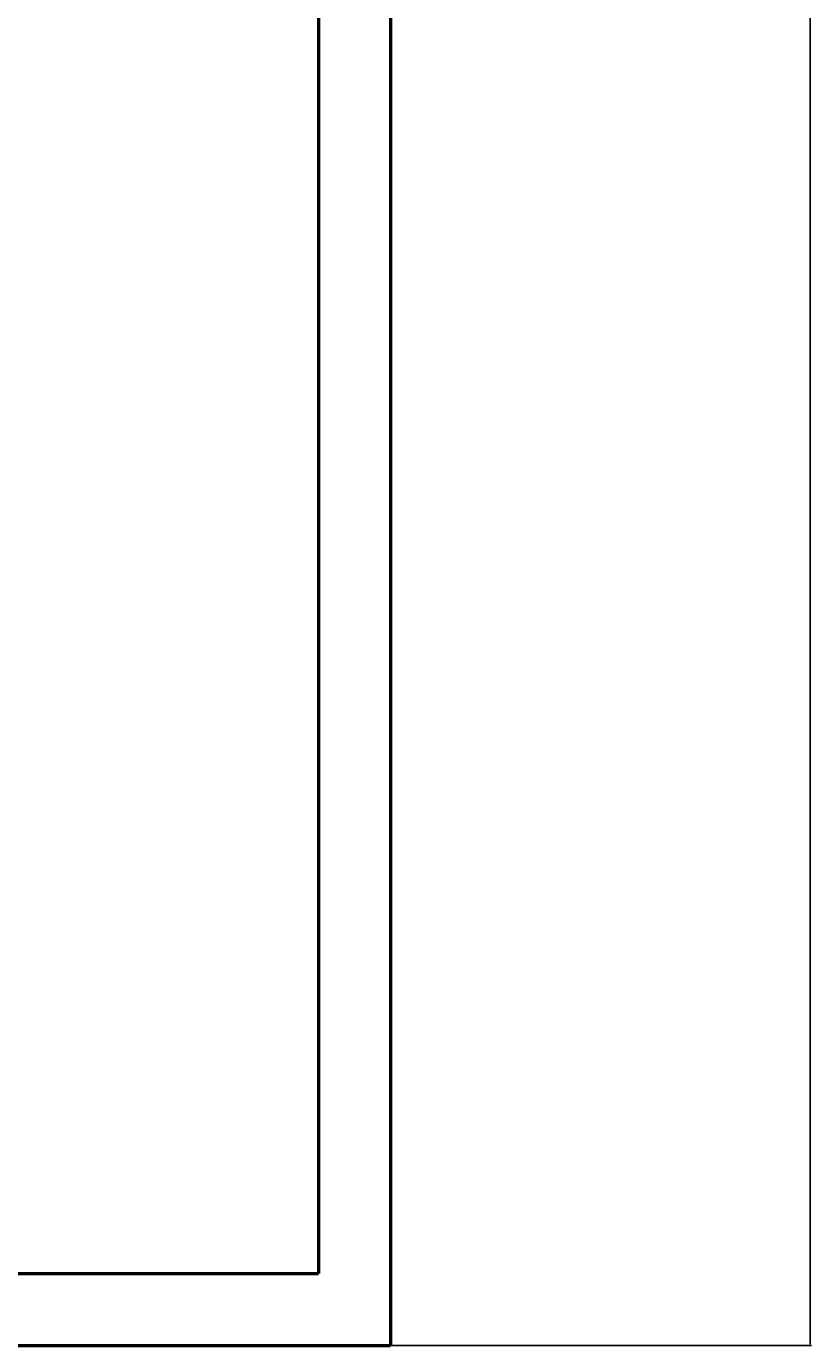
# Model space of a CAD drawing. Units: inches. Extents: x 5375 to 6084, y 16106 to 17259.
# Tile 12 of 32: x 5986 to 6084, y 16212 to 16377. Entities that reach past the tile are written whole.
import ezdxf

# ---------------------------------------------------------------- set-up
doc = ezdxf.new("R2010")
doc.units = ezdxf.units.IN
doc.layers.add('A-ANNO-DIMS', color=2, linetype='Continuous', lineweight=18)
doc.layers.add('WALL', color=6, linetype='Continuous', lineweight=50)
doc.styles.get("Standard").update_dxf_attribs({"font": 'arial.ttf'})
doc.dimstyles.get("Standard").update_dxf_attribs({"dimtxt": 0.18, "dimasz": 0.18, "dimexe": 0.18, "dimexo": 0.0625, "dimgap": 0.09, "dimtad": 0, "dimtih": 1, "dimtoh": 1, "dimdec": 4, "dimzin": 0, "dimdsep": 46, "dimtxsty": 'Standard', "dimcen": 0.09, "dimadec": 0, "dimazin": 0, "dimtfac": 1, "dimtdec": 4, "dimtofl": 0, "dimtmove": 0, "dimatfit": 3, "dimfxl": 1, "dimtolj": 1, "dimtzin": 0, "dimarcsym": 0})

# ---------------------------------------------------------------- blocks, each defined once
blk = doc.blocks.new('*D31')
at = {"layer": 'A-ANNO-DIMS', "color": 0, "lineweight": -2, "transparency": 16777216}
for p, q in [((6031.68, 17206.58), (6084.2, 17206.58)), ((6084.02, 17206.4), (6084.02, 16709.66)), ((6084.02, 16212.56), (6084.02, 16709.3)), ((6031.68, 16212.38), (6084.2, 16212.38))]:
    blk.add_line(p, q, dxfattribs=at)
at = {"layer": 'A-ANNO-DIMS', "color": 0, "transparency": 16777216}
for points in [[(6083.99, 17206.4), (6084.05, 17206.4), (6084.02, 17206.58)], [(6083.99, 16212.56), (6084.05, 16212.56), (6084.02, 16212.38)]]:
    blk.add_solid(points, dxfattribs=at)
at = {"layer": 'Defpoints', "color": 0, "transparency": 16777216}
for p in [(6031.62, 17206.58), (6084.02, 17206.58), (6031.62, 16212.38)]:
    blk.add_point(p, dxfattribs=at)
at = {"layer": 'A-ANNO-DIMS', "color": 0, "transparency": 16777216, "insert": (6084.02, 16709.48), "char_height": 0.18, "attachment_point": 5}
blk.add_mtext('\\A1;994.2', dxfattribs=at)

msp = doc.modelspace()

# ---------------------------------------------------------------- linework, layer by layer
at = {"layer": 'WALL'}
for p, q in [((6031.6199, 16699.5793), (6031.6199, 16212.3785)), ((6022.6199, 16402.5793), (6022.6199, 16221.3785)), ((5479.6199, 16221.3785), (6022.6199, 16221.3785)), ((5470.6199, 16212.3785), (6031.6199, 16212.3785))]:
    msp.add_line(p, q, dxfattribs=at)

# ---------------------------------------------------------------- dimensions: what is measured, and where the dimension line sits
at = {"layer": 'A-ANNO-DIMS'}
dim = msp.add_linear_dim(base=(6084.0199, 17206.5793), p1=(6031.6199, 16212.3785), p2=(6031.6199, 17206.5793), angle=90, dimstyle='Standard', override={"dimdec": 1, "dimlfac": 1, "dimrnd": 0, "dimzin": 0, "dimdsep": 46, "dimlunit": 2}, dxfattribs=at)
dim.commit()
dim.dimension.update_dxf_attribs({"geometry": '*D31', "text_midpoint": (6084.0199, 16709.4789)})

doc.saveas('drawing.dxf')
